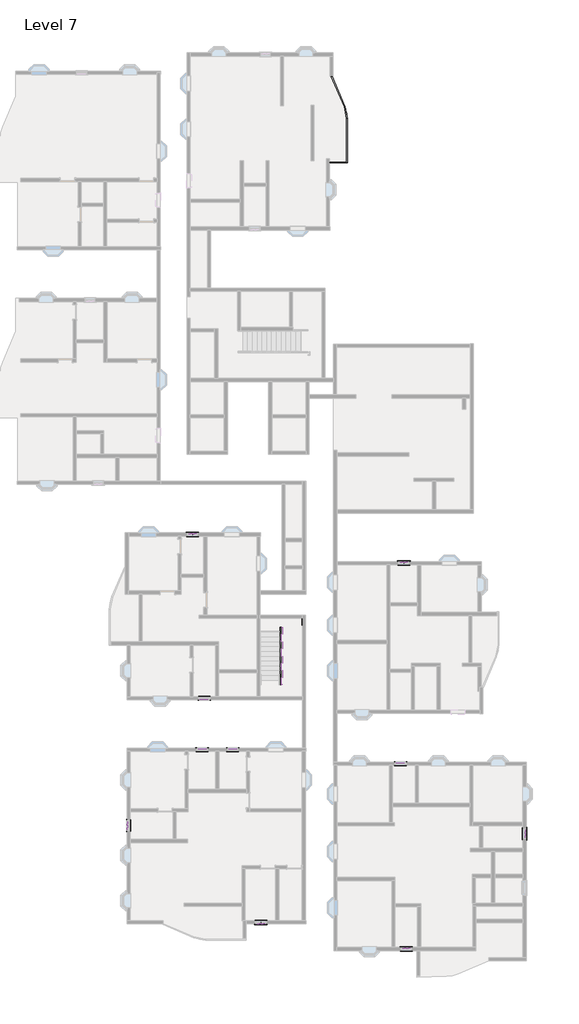
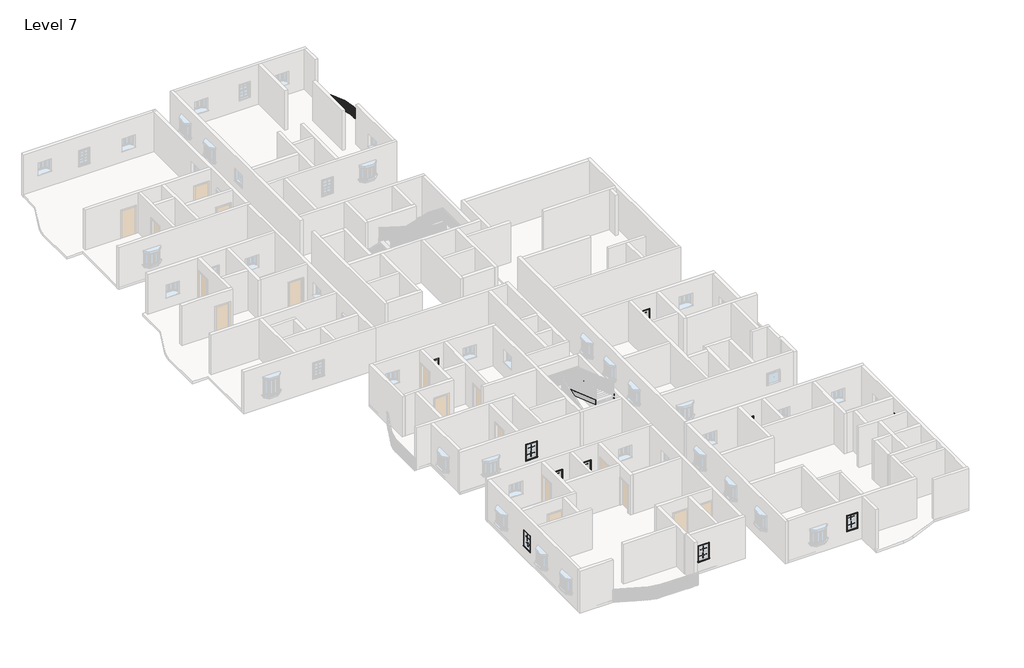
# One storey, part 13 of 14: 40 proxies, 6 members, 1 railing.
"""IFC4 building model written with IfcOpenShell, lengths in millimetres."""

from ifc_helpers import new_model, si_unit, frame, origin, place, context, project, spatial, polyline, circle_curve, outline, extrude, transform, mapped, element, save
from ifc_brep_helpers import plane_surface, cylinder_surface, revolved_surface, advanced_brep
from components import muntin_pattern_2x2_muntin_pattern_2x2_c35c595f, trim_window_exterior_flat_with_sill_e38017c9, trim_window_interior_flat_picture_frame_d728ed12

model = new_model("IFC4")

# Units and contexts
model_context = context("Model", 3, world=origin())
ifc_project = project(units=[si_unit("LENGTHUNIT", "METRE", prefix="MILLI")], contexts=[model_context])

# Site, building, storey
site = spatial("IfcSite", under=ifc_project)
building = spatial("IfcBuilding", under=site)
storey = spatial("IfcBuildingStorey", under=building, Name="Level 7", Elevation=18288.0)

# Proxies
placement = place(None, origin())
muntin_pattern_2x2_muntin_pattern_2x2_shape = muntin_pattern_2x2_muntin_pattern_2x2_c35c595f(model_context)
element("IfcBuildingElementProxy", 1, Name="Muntin Pattern_2x2 : Muntin Pattern_2x2", ObjectType="Muntin Pattern_2x2 : Muntin Pattern_2x2", at=placement, inside=storey, context=model_context, shape_type="MappedRepresentation", body=[
    mapped(muntin_pattern_2x2_muntin_pattern_2x2_shape, transform((-8150.287215, -357.5666506, 19758.025), x_axis=(1.0, 0.0, 0.0), y_axis=(0.0, 1.0, 0.0), z_axis=(0.0, 0.0, 1.0))),
])
element("IfcBuildingElementProxy", 2, Name="Muntin Pattern_2x2 : Muntin Pattern_2x2", ObjectType="Muntin Pattern_2x2 : Muntin Pattern_2x2", at=placement, inside=storey, context=model_context, shape_type="MappedRepresentation", body=[
    mapped(muntin_pattern_2x2_muntin_pattern_2x2_shape, transform((-8150.287215, -402.0166506, 19278.6), x_axis=(1.0, 0.0, 0.0), y_axis=(0.0, 1.0, 0.0), z_axis=(0.0, 0.0, 1.0))),
])
element("IfcBuildingElementProxy", 3, Name="Muntin Pattern_2x2 : Muntin Pattern_2x2", ObjectType="Muntin Pattern_2x2 : Muntin Pattern_2x2", at=placement, inside=storey, context=model_context, shape_type="MappedRepresentation", body=[
    mapped(muntin_pattern_2x2_muntin_pattern_2x2_shape, transform((-7397.812215, -10854.1166506, 19758.025), x_axis=(-1.0, 0.0, 0.0), y_axis=(0.0, -1.0, 0.0), z_axis=(0.0, 0.0, 1.0))),
])
element("IfcBuildingElementProxy", 4, Name="Muntin Pattern_2x2 : Muntin Pattern_2x2", ObjectType="Muntin Pattern_2x2 : Muntin Pattern_2x2", at=placement, inside=storey, context=model_context, shape_type="MappedRepresentation", body=[
    mapped(muntin_pattern_2x2_muntin_pattern_2x2_shape, transform((-7397.812215, -10809.6666506, 19278.6), x_axis=(-1.0, 0.0, 0.0), y_axis=(0.0, -1.0, 0.0), z_axis=(0.0, 0.0, 1.0))),
])
element("IfcBuildingElementProxy", 5, Name="Muntin Pattern_2x2 : Muntin Pattern_2x2", ObjectType="Muntin Pattern_2x2 : Muntin Pattern_2x2", at=placement, inside=storey, context=model_context, shape_type="MappedRepresentation", body=[
    mapped(muntin_pattern_2x2_muntin_pattern_2x2_shape, transform((-7540.687215, -13997.3666506, 19758.025), x_axis=(1.0, 0.0, 0.0), y_axis=(0.0, 1.0, 0.0), z_axis=(0.0, 0.0, 1.0))),
])
element("IfcBuildingElementProxy", 6, Name="Muntin Pattern_2x2 : Muntin Pattern_2x2", ObjectType="Muntin Pattern_2x2 : Muntin Pattern_2x2", at=placement, inside=storey, context=model_context, shape_type="MappedRepresentation", body=[
    mapped(muntin_pattern_2x2_muntin_pattern_2x2_shape, transform((-7540.687215, -14041.8166506, 19278.6), x_axis=(1.0, 0.0, 0.0), y_axis=(0.0, 1.0, 0.0), z_axis=(0.0, 0.0, 1.0))),
])
element("IfcBuildingElementProxy", 7, Name="Muntin Pattern_2x2 : Muntin Pattern_2x2", ObjectType="Muntin Pattern_2x2 : Muntin Pattern_2x2", at=placement, inside=storey, context=model_context, shape_type="MappedRepresentation", body=[
    mapped(muntin_pattern_2x2_muntin_pattern_2x2_shape, transform((-5597.587215, -13997.3666506, 19758.025), x_axis=(1.0, 0.0, 0.0), y_axis=(0.0, 1.0, 0.0), z_axis=(0.0, 0.0, 1.0))),
])
element("IfcBuildingElementProxy", 8, Name="Muntin Pattern_2x2 : Muntin Pattern_2x2", ObjectType="Muntin Pattern_2x2 : Muntin Pattern_2x2", at=placement, inside=storey, context=model_context, shape_type="MappedRepresentation", body=[
    mapped(muntin_pattern_2x2_muntin_pattern_2x2_shape, transform((-5597.587215, -14041.8166506, 19278.6), x_axis=(1.0, 0.0, 0.0), y_axis=(0.0, 1.0, 0.0), z_axis=(0.0, 0.0, 1.0))),
])
element("IfcBuildingElementProxy", 9, Name="Muntin Pattern_2x2 : Muntin Pattern_2x2", ObjectType="Muntin Pattern_2x2 : Muntin Pattern_2x2", at=placement, inside=storey, context=model_context, shape_type="MappedRepresentation", body=[
    mapped(muntin_pattern_2x2_muntin_pattern_2x2_shape, transform((-12255.562215, -18863.6994419, 19758.025), x_axis=(0.0, 1.0, 0.0), y_axis=(-1.0, 0.0, 0.0), z_axis=(0.0, 0.0, 1.0))),
])
element("IfcBuildingElementProxy", 10, Name="Muntin Pattern_2x2 : Muntin Pattern_2x2", ObjectType="Muntin Pattern_2x2 : Muntin Pattern_2x2", at=placement, inside=storey, context=model_context, shape_type="MappedRepresentation", body=[
    mapped(muntin_pattern_2x2_muntin_pattern_2x2_shape, transform((-12211.112215, -18863.6994419, 19278.6), x_axis=(0.0, 1.0, 0.0), y_axis=(-1.0, 0.0, 0.0), z_axis=(0.0, 0.0, 1.0))),
])
element("IfcBuildingElementProxy", 11, Name="Muntin Pattern_2x2 : Muntin Pattern_2x2", ObjectType="Muntin Pattern_2x2 : Muntin Pattern_2x2", at=placement, inside=storey, context=model_context, shape_type="MappedRepresentation", body=[
    mapped(muntin_pattern_2x2_muntin_pattern_2x2_shape, transform((-3806.2891351, -25065.4166506, 19758.025), x_axis=(-1.0, 0.0, 0.0), y_axis=(0.0, -1.0, 0.0), z_axis=(0.0, 0.0, 1.0))),
])
element("IfcBuildingElementProxy", 12, Name="Muntin Pattern_2x2 : Muntin Pattern_2x2", ObjectType="Muntin Pattern_2x2 : Muntin Pattern_2x2", at=placement, inside=storey, context=model_context, shape_type="MappedRepresentation", body=[
    mapped(muntin_pattern_2x2_muntin_pattern_2x2_shape, transform((-3806.2891351, -25020.9666506, 19278.6), x_axis=(-1.0, 0.0, 0.0), y_axis=(0.0, -1.0, 0.0), z_axis=(0.0, 0.0, 1.0))),
])
element("IfcBuildingElementProxy", 13, Name="Muntin Pattern_2x2 : Muntin Pattern_2x2", ObjectType="Muntin Pattern_2x2 : Muntin Pattern_2x2", at=placement, inside=storey, context=model_context, shape_type="MappedRepresentation", body=[
    mapped(muntin_pattern_2x2_muntin_pattern_2x2_shape, transform((5410.0380523, -26615.6292694, 19758.025), x_axis=(1.0, 0.0, 0.0), y_axis=(0.0, 1.0, 0.0), z_axis=(0.0, 0.0, 1.0))),
])
element("IfcBuildingElementProxy", 14, Name="Muntin Pattern_2x2 : Muntin Pattern_2x2", ObjectType="Muntin Pattern_2x2 : Muntin Pattern_2x2", at=placement, inside=storey, context=model_context, shape_type="MappedRepresentation", body=[
    mapped(muntin_pattern_2x2_muntin_pattern_2x2_shape, transform((5410.0380523, -26660.0792694, 19278.6), x_axis=(1.0, 0.0, 0.0), y_axis=(0.0, 1.0, 0.0), z_axis=(0.0, 0.0, 1.0))),
])
element("IfcBuildingElementProxy", 15, Name="Muntin Pattern_2x2 : Muntin Pattern_2x2", ObjectType="Muntin Pattern_2x2 : Muntin Pattern_2x2", at=placement, inside=storey, context=model_context, shape_type="MappedRepresentation", body=[
    mapped(muntin_pattern_2x2_muntin_pattern_2x2_shape, transform((12982.4130523, -19379.8042694, 19758.025), x_axis=(0.0, -1.0, 0.0), y_axis=(1.0, 0.0, 0.0), z_axis=(0.0, 0.0, 1.0))),
])
element("IfcBuildingElementProxy", 16, Name="Muntin Pattern_2x2 : Muntin Pattern_2x2", ObjectType="Muntin Pattern_2x2 : Muntin Pattern_2x2", at=placement, inside=storey, context=model_context, shape_type="MappedRepresentation", body=[
    mapped(muntin_pattern_2x2_muntin_pattern_2x2_shape, transform((12937.9630523, -19379.8042694, 19278.6), x_axis=(0.0, -1.0, 0.0), y_axis=(1.0, 0.0, 0.0), z_axis=(0.0, 0.0, 1.0))),
])
element("IfcBuildingElementProxy", 17, Name="Muntin Pattern_2x2 : Muntin Pattern_2x2", ObjectType="Muntin Pattern_2x2 : Muntin Pattern_2x2", at=placement, inside=storey, context=model_context, shape_type="MappedRepresentation", body=[
    mapped(muntin_pattern_2x2_muntin_pattern_2x2_shape, transform((5048.0880523, -14880.8292694, 19758.025), x_axis=(1.0, 0.0, 0.0), y_axis=(0.0, 1.0, 0.0), z_axis=(0.0, 0.0, 1.0))),
])
element("IfcBuildingElementProxy", 18, Name="Muntin Pattern_2x2 : Muntin Pattern_2x2", ObjectType="Muntin Pattern_2x2 : Muntin Pattern_2x2", at=placement, inside=storey, context=model_context, shape_type="MappedRepresentation", body=[
    mapped(muntin_pattern_2x2_muntin_pattern_2x2_shape, transform((5048.0880523, -14925.2792694, 19278.6), x_axis=(1.0, 0.0, 0.0), y_axis=(0.0, 1.0, 0.0), z_axis=(0.0, 0.0, 1.0))),
])
element("IfcBuildingElementProxy", 19, Name="Muntin Pattern_2x2 : Muntin Pattern_2x2", ObjectType="Muntin Pattern_2x2 : Muntin Pattern_2x2", at=placement, inside=storey, context=model_context, shape_type="MappedRepresentation", body=[
    mapped(muntin_pattern_2x2_muntin_pattern_2x2_shape, transform((5257.6380523, -2168.1292694, 19758.025), x_axis=(1.0, 0.0, 0.0), y_axis=(0.0, 1.0, 0.0), z_axis=(0.0, 0.0, 1.0))),
])
element("IfcBuildingElementProxy", 20, Name="Muntin Pattern_2x2 : Muntin Pattern_2x2", ObjectType="Muntin Pattern_2x2 : Muntin Pattern_2x2", at=placement, inside=storey, context=model_context, shape_type="MappedRepresentation", body=[
    mapped(muntin_pattern_2x2_muntin_pattern_2x2_shape, transform((5257.6380523, -2212.5792694, 19278.6), x_axis=(1.0, 0.0, 0.0), y_axis=(0.0, 1.0, 0.0), z_axis=(0.0, 0.0, 1.0))),
])
trim_window_exterior_flat_with_sill_shape = trim_window_exterior_flat_with_sill_e38017c9(model_context)
element("IfcBuildingElementProxy", 21, Name="Trim-Window-Exterior-Flat : with Sill", ObjectType="Trim-Window-Exterior-Flat : with Sill", at=placement, inside=storey, context=model_context, shape_type="MappedRepresentation", body=[
    mapped(trim_window_exterior_flat_with_sill_shape, transform((-8150.287215, -322.6416506, 20269.2), x_axis=(-1.0, 0.0, 0.0), y_axis=(0.0, 0.0, 1.0), z_axis=(0.0, 1.0, 0.0))),
])
element("IfcBuildingElementProxy", 22, Name="Trim-Window-Exterior-Flat : with Sill", ObjectType="Trim-Window-Exterior-Flat : with Sill", at=placement, inside=storey, context=model_context, shape_type="MappedRepresentation", body=[
    mapped(trim_window_exterior_flat_with_sill_shape, transform((-7397.812215, -10889.0416506, 20269.2), x_axis=(1.0, 0.0, 0.0), y_axis=(0.0, 0.0, 1.0), z_axis=(0.0, -1.0, 0.0))),
])
element("IfcBuildingElementProxy", 23, Name="Trim-Window-Exterior-Flat : with Sill", ObjectType="Trim-Window-Exterior-Flat : with Sill", at=placement, inside=storey, context=model_context, shape_type="MappedRepresentation", body=[
    mapped(trim_window_exterior_flat_with_sill_shape, transform((-7540.687215, -13962.4416506, 20269.2), x_axis=(-1.0, 0.0, 0.0), y_axis=(0.0, 0.0, 1.0), z_axis=(0.0, 1.0, 0.0))),
])
element("IfcBuildingElementProxy", 24, Name="Trim-Window-Exterior-Flat : with Sill", ObjectType="Trim-Window-Exterior-Flat : with Sill", at=placement, inside=storey, context=model_context, shape_type="MappedRepresentation", body=[
    mapped(trim_window_exterior_flat_with_sill_shape, transform((-5597.587215, -13962.4416506, 20269.2), x_axis=(-1.0, 0.0, 0.0), y_axis=(0.0, 0.0, 1.0), z_axis=(0.0, 1.0, 0.0))),
])
element("IfcBuildingElementProxy", 25, Name="Trim-Window-Exterior-Flat : with Sill", ObjectType="Trim-Window-Exterior-Flat : with Sill", at=placement, inside=storey, context=model_context, shape_type="MappedRepresentation", body=[
    mapped(trim_window_exterior_flat_with_sill_shape, transform((-12290.487215, -18863.6994419, 20269.2), x_axis=(0.0, -1.0, 0.0), y_axis=(0.0, 0.0, 1.0), z_axis=(-1.0, 0.0, 0.0))),
])
element("IfcBuildingElementProxy", 26, Name="Trim-Window-Exterior-Flat : with Sill", ObjectType="Trim-Window-Exterior-Flat : with Sill", at=placement, inside=storey, context=model_context, shape_type="MappedRepresentation", body=[
    mapped(trim_window_exterior_flat_with_sill_shape, transform((-3806.2891351, -25100.3416506, 20269.2), x_axis=(1.0, 0.0, 0.0), y_axis=(0.0, 0.0, 1.0), z_axis=(0.0, -1.0, 0.0))),
])
element("IfcBuildingElementProxy", 27, Name="Trim-Window-Exterior-Flat : with Sill", ObjectType="Trim-Window-Exterior-Flat : with Sill", at=placement, inside=storey, context=model_context, shape_type="MappedRepresentation", body=[
    mapped(trim_window_exterior_flat_with_sill_shape, transform((5410.0380523, -26580.7042694, 20269.2), x_axis=(-1.0, 0.0, 0.0), y_axis=(0.0, 0.0, 1.0), z_axis=(0.0, 1.0, 0.0))),
])
element("IfcBuildingElementProxy", 28, Name="Trim-Window-Exterior-Flat : with Sill", ObjectType="Trim-Window-Exterior-Flat : with Sill", at=placement, inside=storey, context=model_context, shape_type="MappedRepresentation", body=[
    mapped(trim_window_exterior_flat_with_sill_shape, transform((13017.3380523, -19379.8042694, 20269.2), x_axis=(0.0, 1.0, 0.0), y_axis=(0.0, 0.0, 1.0), z_axis=(1.0, 0.0, 0.0))),
])
element("IfcBuildingElementProxy", 29, Name="Trim-Window-Exterior-Flat : with Sill", ObjectType="Trim-Window-Exterior-Flat : with Sill", at=placement, inside=storey, context=model_context, shape_type="MappedRepresentation", body=[
    mapped(trim_window_exterior_flat_with_sill_shape, transform((5048.0880523, -14845.9042694, 20269.2), x_axis=(-1.0, 0.0, 0.0), y_axis=(0.0, 0.0, 1.0), z_axis=(0.0, 1.0, 0.0))),
])
element("IfcBuildingElementProxy", 30, Name="Trim-Window-Exterior-Flat : with Sill", ObjectType="Trim-Window-Exterior-Flat : with Sill", at=placement, inside=storey, context=model_context, shape_type="MappedRepresentation", body=[
    mapped(trim_window_exterior_flat_with_sill_shape, transform((5257.6380523, -2133.2042694, 20269.2), x_axis=(-1.0, 0.0, 0.0), y_axis=(0.0, 0.0, 1.0), z_axis=(0.0, 1.0, 0.0))),
])
trim_window_interior_flat_picture_frame_shape = trim_window_interior_flat_picture_frame_d728ed12(model_context)
element("IfcBuildingElementProxy", 31, Name="Trim-Window-Interior-Flat : Picture Frame", ObjectType="Trim-Window-Interior-Flat : Picture Frame", at=placement, inside=storey, context=model_context, shape_type="MappedRepresentation", body=[
    mapped(trim_window_interior_flat_picture_frame_shape, transform((-8150.287215, -525.8416506, 20269.2), x_axis=(1.0, 0.0, 0.0), y_axis=(0.0, 0.0, 1.0), z_axis=(0.0, -1.0, 0.0))),
])
element("IfcBuildingElementProxy", 32, Name="Trim-Window-Interior-Flat : Picture Frame", ObjectType="Trim-Window-Interior-Flat : Picture Frame", at=placement, inside=storey, context=model_context, shape_type="MappedRepresentation", body=[
    mapped(trim_window_interior_flat_picture_frame_shape, transform((-7397.812215, -10685.8416506, 20269.2), x_axis=(-1.0, 0.0, 0.0), y_axis=(0.0, 0.0, 1.0), z_axis=(0.0, 1.0, 0.0))),
])
element("IfcBuildingElementProxy", 33, Name="Trim-Window-Interior-Flat : Picture Frame", ObjectType="Trim-Window-Interior-Flat : Picture Frame", at=placement, inside=storey, context=model_context, shape_type="MappedRepresentation", body=[
    mapped(trim_window_interior_flat_picture_frame_shape, transform((-7540.687215, -14165.6416506, 20269.2), x_axis=(1.0, 0.0, 0.0), y_axis=(0.0, 0.0, 1.0), z_axis=(0.0, -1.0, 0.0))),
])
element("IfcBuildingElementProxy", 34, Name="Trim-Window-Interior-Flat : Picture Frame", ObjectType="Trim-Window-Interior-Flat : Picture Frame", at=placement, inside=storey, context=model_context, shape_type="MappedRepresentation", body=[
    mapped(trim_window_interior_flat_picture_frame_shape, transform((-5597.587215, -14165.6416506, 20269.2), x_axis=(1.0, 0.0, 0.0), y_axis=(0.0, 0.0, 1.0), z_axis=(0.0, -1.0, 0.0))),
])
element("IfcBuildingElementProxy", 35, Name="Trim-Window-Interior-Flat : Picture Frame", ObjectType="Trim-Window-Interior-Flat : Picture Frame", at=placement, inside=storey, context=model_context, shape_type="MappedRepresentation", body=[
    mapped(trim_window_interior_flat_picture_frame_shape, transform((-12087.287215, -18863.6994419, 20269.2), x_axis=(0.0, 1.0, 0.0), y_axis=(0.0, 0.0, 1.0), z_axis=(1.0, 0.0, 0.0))),
])
element("IfcBuildingElementProxy", 36, Name="Trim-Window-Interior-Flat : Picture Frame", ObjectType="Trim-Window-Interior-Flat : Picture Frame", at=placement, inside=storey, context=model_context, shape_type="MappedRepresentation", body=[
    mapped(trim_window_interior_flat_picture_frame_shape, transform((-3806.2891351, -24897.1416506, 20269.2), x_axis=(-1.0, 0.0, 0.0), y_axis=(0.0, 0.0, 1.0), z_axis=(0.0, 1.0, 0.0))),
])
element("IfcBuildingElementProxy", 37, Name="Trim-Window-Interior-Flat : Picture Frame", ObjectType="Trim-Window-Interior-Flat : Picture Frame", at=placement, inside=storey, context=model_context, shape_type="MappedRepresentation", body=[
    mapped(trim_window_interior_flat_picture_frame_shape, transform((5410.0380523, -26783.9042694, 20269.2), x_axis=(1.0, 0.0, 0.0), y_axis=(0.0, 0.0, 1.0), z_axis=(0.0, -1.0, 0.0))),
])
element("IfcBuildingElementProxy", 38, Name="Trim-Window-Interior-Flat : Picture Frame", ObjectType="Trim-Window-Interior-Flat : Picture Frame", at=placement, inside=storey, context=model_context, shape_type="MappedRepresentation", body=[
    mapped(trim_window_interior_flat_picture_frame_shape, transform((12814.1380523, -19379.8042694, 20269.2), x_axis=(0.0, -1.0, 0.0), y_axis=(0.0, 0.0, 1.0), z_axis=(-1.0, 0.0, 0.0))),
])
element("IfcBuildingElementProxy", 39, Name="Trim-Window-Interior-Flat : Picture Frame", ObjectType="Trim-Window-Interior-Flat : Picture Frame", at=placement, inside=storey, context=model_context, shape_type="MappedRepresentation", body=[
    mapped(trim_window_interior_flat_picture_frame_shape, transform((5048.0880523, -15049.1042694, 20269.2), x_axis=(1.0, 0.0, 0.0), y_axis=(0.0, 0.0, 1.0), z_axis=(0.0, -1.0, 0.0))),
])
element("IfcBuildingElementProxy", 40, Name="Trim-Window-Interior-Flat : Picture Frame", ObjectType="Trim-Window-Interior-Flat : Picture Frame", at=placement, inside=storey, context=model_context, shape_type="MappedRepresentation", body=[
    mapped(trim_window_interior_flat_picture_frame_shape, transform((5257.6380523, -2336.4042694, 20269.2), x_axis=(1.0, 0.0, 0.0), y_axis=(0.0, 0.0, 1.0), z_axis=(0.0, -1.0, 0.0))),
])

# Members
element("IfcMember", 41, ObjectType="Stringer - 2\" Width", at=placement, inside=storey, context=model_context, shape_type="SweptSolid", body=[
    extrude(outline(polyline([(-9955.5916506, 18288.0), (-9955.5916506, 18479.3592169), (-6325.8738327, 19735.8), (-5713.7916506, 19735.8), (-5713.7916506, 19625.1301656), (-9576.612129, 18288.0), (-9955.5916506, 18288.0)])), frame((-3908.487215, 0.0, 0.0), z_axis=(1.0, 0.0, 0.0), x_axis=(0.0, 1.0, 0.0)), (0.0, 0.0, 1.0), 50.8),
])
element("IfcMember", 42, ObjectType="Stringer - 2\" Width", at=placement, inside=storey, context=model_context, shape_type="SweptSolid", body=[
    extrude(outline(polyline([(-3908.487215, -5713.7916506), (-3908.487215, -5662.9916506), (-1190.687215, -5662.9916506), (-1190.687215, -5713.7916506), (-3908.487215, -5713.7916506)])), frame((0.0, 0.0, 19431.0), z_axis=(0.0, 0.0, 1.0), x_axis=(1.0, 0.0, 0.0)), (0.0, 0.0, 1.0), 304.8),
])
element("IfcMember", 43, ObjectType="Stringer - 2\" Width", at=placement, inside=storey, context=model_context, shape_type="SweptSolid", body=[
    extrude(outline(polyline([(-5662.9916506, 19635.5476784), (-5662.9916506, 19431.0), (-6003.8711722, 19431.0), (-9949.2416506, 20796.7051656), (-9949.2416506, 21119.2496015), (-5662.9916506, 19635.5476784)])), frame((-1190.687215, 0.0, 0.0), z_axis=(1.0, 0.0, 0.0), x_axis=(0.0, 1.0, 0.0)), (0.0, 0.0, 1.0), 50.8),
])
element("IfcMember", 44, ObjectType="Stringer - 2\" Width", at=placement, inside=storey, context=model_context, shape_type="SweptSolid", body=[
    extrude(outline(polyline([(-9955.5916506, 18288.0), (-9955.5916506, 18479.3592169), (-6342.4416506, 19730.0649861), (-6342.4416506, 19407.5205502), (-9576.612129, 18288.0), (-9955.5916506, 18288.0)])), frame((-2593.7381751, 0.0, 0.0), z_axis=(1.0, 0.0, 0.0), x_axis=(0.0, 1.0, 0.0)), (0.0, 0.0, 1.0), 50.8),
])
element("IfcMember", 45, ObjectType="Stringer - 2\" Width", at=placement, inside=storey, context=model_context, shape_type="SweptSolid", body=[
    extrude(outline(polyline([(-2593.7381751, -6342.4416506), (-2593.7381751, -6291.6416506), (-2492.1381751, -6291.6416506), (-2492.1381751, -6342.4416506), (-2593.7381751, -6342.4416506)])), frame((0.0, 0.0, 19431.0), z_axis=(0.0, 0.0, 1.0), x_axis=(1.0, 0.0, 0.0)), (0.0, 0.0, 1.0), 304.8),
])
element("IfcMember", 46, ObjectType="Stringer - 2\" Width", at=placement, inside=storey, context=model_context, shape_type="SweptSolid", body=[
    extrude(outline(polyline([(-6291.6416506, 19853.1572938), (-6291.6416506, 19530.6128579), (-9949.2416506, 20796.7051656), (-9949.2416506, 21119.2496015), (-6291.6416506, 19853.1572938)])), frame((-2492.1381751, 0.0, 0.0), z_axis=(1.0, 0.0, 0.0), x_axis=(0.0, 1.0, 0.0)), (0.0, 0.0, 1.0), 50.8),
])

# Railing
element("IfcRailing", 47, ObjectType="Handrail - Rectangular", at=placement, inside=storey, context=model_context, shape_type="SolidModel", body=[
    advanced_brep(
    [(549.8108649, 23180.4215905, 19202.4), (549.8108649, 23180.4215905, 19151.6), (549.8108649, 23129.6215905, 19151.6), (549.8108649, 23129.6215905, 19202.4), (1629.3108649, 23180.4215905, 19202.4), (1629.3108649, 23180.4215905, 19151.6), (1680.1108649, 23129.6215905, 19151.6), (1680.1108649, 23129.6215905, 19202.4), (1629.3108649, 25921.9580583, 19202.4), (1629.3108649, 25921.9580583, 19151.6), (1680.1108649, 25921.9580583, 19151.6), (1680.1108649, 25921.9580583, 19202.4), (1475.5051478, 26671.8537734, 19151.6), (1475.5051478, 26671.8537734, 19202.4), (1522.203662, 26691.8509925, 19151.6), (1522.203662, 26691.8509925, 19202.4), (640.7616078, 28621.188975, 19202.4), (687.460122, 28641.186194, 19202.4), (687.460122, 28641.186194, 19151.6), (640.7616078, 28621.188975, 19151.6)],
    [
        (0, 1),
        (1, 2),
        (2, 3),
        (3, 0),
        (0, 4),
        (4, 5),
        (5, 1),
        (5, 6),
        (6, 2),
        (6, 7),
        (7, 3),
        (7, 4),
        (4, 8),
        (8, 9),
        (9, 5),
        (9, 10),
        (10, 6),
        (10, 11),
        (11, 7),
        (11, 8),
        (12, 9, circle_curve(frame((-275.6891351, 25921.9580583, 19151.6), z_axis=(0.0, 0.0, -1.0), x_axis=(1.0, 0.0, 0.0)), 1905.0)),
        (8, 13, circle_curve(frame((-275.6891351, 25921.9580583, 19202.4), z_axis=(0.0, 0.0, 1.0), x_axis=(1.0, 0.0, 0.0)), 1905.0)),
        (13, 12),
        (14, 10, circle_curve(frame((-275.6891351, 25921.9580583, 19151.6), z_axis=(0.0, 0.0, -1.0), x_axis=(1.0, 0.0, 0.0)), 1955.8)),
        (12, 14),
        (15, 11, circle_curve(frame((-275.6891351, 25921.9580583, 19202.4), z_axis=(0.0, 0.0, -1.0), x_axis=(1.0, 0.0, 0.0)), 1955.8)),
        (14, 15),
        (15, 13),
        (16, 17),
        (17, 18),
        (18, 19),
        (19, 16),
        (13, 16),
        (19, 12),
        (18, 14),
        (17, 15),
    ],
    [
        plane_surface(frame((549.8108649, 23155.0215905, 19202.4), z_axis=(-1.0, 0.0, 0.0), x_axis=(0.0, 1.0, 0.0))),
        plane_surface(frame((549.8108649, 23180.4215905, 19202.4), z_axis=(0.0, 1.0, 0.0), x_axis=(1.0, 0.0, 0.0))),
        plane_surface(frame((549.8108649, 23180.4215905, 19151.6), z_axis=(0.0, 0.0, -1.0), x_axis=(1.0, 0.0, 0.0))),
        plane_surface(frame((549.8108649, 23129.6215905, 19151.6), z_axis=(0.0, -1.0, 0.0), x_axis=(1.0, 0.0, 0.0))),
        plane_surface(frame((549.8108649, 23129.6215905, 19202.4), z_axis=(0.0, 0.0, 1.0), x_axis=(1.0, 0.0, 0.0))),
        plane_surface(frame((1629.3108649, 23180.4215905, 19202.4), z_axis=(-1.0, 0.0, 0.0), x_axis=(0.0, 1.0, 0.0))),
        plane_surface(frame((1629.3108649, 23180.4215905, 19151.6), z_axis=(0.0, 0.0, -1.0), x_axis=(0.0, 1.0, 0.0))),
        plane_surface(frame((1680.1108649, 23129.6215905, 19151.6), z_axis=(1.0, 0.0, 0.0), x_axis=(0.0, 1.0, 0.0))),
        plane_surface(frame((1680.1108649, 23129.6215905, 19202.4), z_axis=(0.0, 0.0, 1.0), x_axis=(0.0, 1.0, 0.0))),
        revolved_surface(polyline([(1629.3108649, 25921.9580583, 19202.4), (1629.3108649, 25921.9580583, 19151.6)]), (-275.6891351, 25921.9580583, 19202.4), (0.0, 0.0, 1.0)),
        plane_surface(frame((-275.6891351, 25921.9580583, 19151.6), z_axis=(0.0, 0.0, -1.0), x_axis=(1.0, 0.0, 0.0))),
        cylinder_surface(frame((-275.6891351, 25921.9580583, 19202.4), z_axis=(0.0, 0.0, 1.0), x_axis=(1.0, 0.0, 0.0)), 1955.8),
        plane_surface(frame((-275.6891351, 25921.9580583, 19202.4), z_axis=(0.0, 0.0, 1.0), x_axis=(1.0, 0.0, 0.0))),
        plane_surface(frame((664.1108649, 28631.1875845, 19202.4), z_axis=(-0.39364604467361036, 0.91926209076238, 0.0), x_axis=(0.91926209076238, 0.39364604467361036, 0.0))),
        plane_surface(frame((1475.5051478, 26671.8537734, 19202.4), z_axis=(-0.91926209076238, -0.3936460446736102, 0.0), x_axis=(-0.3936460446736102, 0.91926209076238, 0.0))),
        plane_surface(frame((1475.5051478, 26671.8537734, 19151.6), z_axis=(0.0, 0.0, -1.0), x_axis=(-0.3936460446736102, 0.91926209076238, 0.0))),
        plane_surface(frame((1522.203662, 26691.8509925, 19151.6), z_axis=(0.91926209076238, 0.3936460446736102, 0.0), x_axis=(-0.3936460446736102, 0.91926209076238, 0.0))),
        plane_surface(frame((1522.203662, 26691.8509925, 19202.4), z_axis=(0.0, 0.0, 1.0), x_axis=(-0.3936460446736102, 0.91926209076238, 0.0))),
    ],
    [
        (0, [[1, 2, 3, 4]]),
        (1, [[-1, 5, 6, 7]]),
        (2, [[-2, -7, 8, 9]]),
        (3, [[-3, -9, 10, 11]]),
        (4, [[-4, -11, 12, -5]]),
        (5, [[-6, 13, 14, 15]]),
        (6, [[-8, -15, 16, 17]]),
        (7, [[-10, -17, 18, 19]]),
        (8, [[-12, -19, 20, -13]]),
        (9, [[21, -14, 22, 23]]),
        (10, [[24, -16, -21, 25]]),
        (11, [[26, -18, -24, 27]]),
        (12, [[-22, -20, -26, 28]]),
        (13, [[29, 30, 31, 32]]),
        (14, [[-23, 33, -32, 34]]),
        (15, [[-25, -34, -31, 35]]),
        (16, [[-27, -35, -30, 36]]),
        (17, [[-28, -36, -29, -33]]),
    ],
),
    extrude(outline(polyline([(711.4710921, 28544.7864585), (693.9591493, 28537.2875014), (686.4601921, 28554.7994442), (703.9721349, 28562.2984014), (711.4710921, 28544.7864585)])), frame((0.0, 0.0, 18288.0), z_axis=(0.0, 0.0, 1.0), x_axis=(1.0, 0.0, 0.0)), (0.0, 0.0, 1.0), 863.6),
    extrude(outline(polyline([(751.4655302, 28451.3894301), (733.9535874, 28443.890473), (726.4546303, 28461.4024158), (743.9665731, 28468.9013729), (751.4655302, 28451.3894301)])), frame((0.0, 0.0, 18288.0), z_axis=(0.0, 0.0, 1.0), x_axis=(1.0, 0.0, 0.0)), (0.0, 0.0, 1.0), 863.6),
    extrude(outline(polyline([(791.4599684, 28357.9924017), (773.9480255, 28350.4934445), (766.4490684, 28368.0053874), (783.9610112, 28375.5043445), (791.4599684, 28357.9924017)])), frame((0.0, 0.0, 18288.0), z_axis=(0.0, 0.0, 1.0), x_axis=(1.0, 0.0, 0.0)), (0.0, 0.0, 1.0), 863.6),
    extrude(outline(polyline([(831.4544065, 28264.5953733), (813.9424637, 28257.0964161), (806.4435065, 28274.608359), (823.9554494, 28282.1073161), (831.4544065, 28264.5953733)])), frame((0.0, 0.0, 18288.0), z_axis=(0.0, 0.0, 1.0), x_axis=(1.0, 0.0, 0.0)), (0.0, 0.0, 1.0), 863.6),
    extrude(outline(polyline([(871.4488446, 28171.1983449), (853.9369018, 28163.6993877), (846.4379447, 28181.2113305), (863.9498875, 28188.7102877), (871.4488446, 28171.1983449)])), frame((0.0, 0.0, 18288.0), z_axis=(0.0, 0.0, 1.0), x_axis=(1.0, 0.0, 0.0)), (0.0, 0.0, 1.0), 863.6),
    extrude(outline(polyline([(911.4432828, 28077.8013164), (893.93134, 28070.3023593), (886.4323828, 28087.8143021), (903.9443256, 28095.3132593), (911.4432828, 28077.8013164)])), frame((0.0, 0.0, 18288.0), z_axis=(0.0, 0.0, 1.0), x_axis=(1.0, 0.0, 0.0)), (0.0, 0.0, 1.0), 863.6),
    extrude(outline(polyline([(951.4377209, 27984.404288), (933.9257781, 27976.9053309), (926.4268209, 27994.4172737), (943.9387638, 28001.9162308), (951.4377209, 27984.404288)])), frame((0.0, 0.0, 18288.0), z_axis=(0.0, 0.0, 1.0), x_axis=(1.0, 0.0, 0.0)), (0.0, 0.0, 1.0), 863.6),
    extrude(outline(polyline([(991.4321591, 27891.0072596), (973.9202162, 27883.5083024), (966.4212591, 27901.0202453), (983.9332019, 27908.5192024), (991.4321591, 27891.0072596)])), frame((0.0, 0.0, 18288.0), z_axis=(0.0, 0.0, 1.0), x_axis=(1.0, 0.0, 0.0)), (0.0, 0.0, 1.0), 863.6),
    extrude(outline(polyline([(1031.4265972, 27797.6102312), (1013.9146544, 27790.111274), (1006.4156972, 27807.6232168), (1023.9276401, 27815.122174), (1031.4265972, 27797.6102312)])), frame((0.0, 0.0, 18288.0), z_axis=(0.0, 0.0, 1.0), x_axis=(1.0, 0.0, 0.0)), (0.0, 0.0, 1.0), 863.6),
    extrude(outline(polyline([(1071.4210353, 27704.2132027), (1053.9090925, 27696.7142456), (1046.4101354, 27714.2261884), (1063.9220782, 27721.7251456), (1071.4210353, 27704.2132027)])), frame((0.0, 0.0, 18288.0), z_axis=(0.0, 0.0, 1.0), x_axis=(1.0, 0.0, 0.0)), (0.0, 0.0, 1.0), 863.6),
    extrude(outline(polyline([(1111.4154735, 27610.8161743), (1093.9035307, 27603.3172172), (1086.4045735, 27620.82916), (1103.9165163, 27628.3281172), (1111.4154735, 27610.8161743)])), frame((0.0, 0.0, 18288.0), z_axis=(0.0, 0.0, 1.0), x_axis=(1.0, 0.0, 0.0)), (0.0, 0.0, 1.0), 863.6),
    extrude(outline(polyline([(1151.4099116, 27517.4191459), (1133.8979688, 27509.9201888), (1126.3990116, 27527.4321316), (1143.9109545, 27534.9310887), (1151.4099116, 27517.4191459)])), frame((0.0, 0.0, 18288.0), z_axis=(0.0, 0.0, 1.0), x_axis=(1.0, 0.0, 0.0)), (0.0, 0.0, 1.0), 863.6),
    extrude(outline(polyline([(1191.4043498, 27424.0221175), (1173.8924069, 27416.5231603), (1166.3934498, 27434.0351032), (1183.9053926, 27441.5340603), (1191.4043498, 27424.0221175)])), frame((0.0, 0.0, 18288.0), z_axis=(0.0, 0.0, 1.0), x_axis=(1.0, 0.0, 0.0)), (0.0, 0.0, 1.0), 863.6),
    extrude(outline(polyline([(1231.3987879, 27330.6250891), (1213.8868451, 27323.1261319), (1206.3878879, 27340.6380747), (1223.8998307, 27348.1370319), (1231.3987879, 27330.6250891)])), frame((0.0, 0.0, 18288.0), z_axis=(0.0, 0.0, 1.0), x_axis=(1.0, 0.0, 0.0)), (0.0, 0.0, 1.0), 863.6),
    extrude(outline(polyline([(1271.393226, 27237.2280606), (1253.8812832, 27229.7291035), (1246.3823261, 27247.2410463), (1263.8942689, 27254.7400035), (1271.393226, 27237.2280606)])), frame((0.0, 0.0, 18288.0), z_axis=(0.0, 0.0, 1.0), x_axis=(1.0, 0.0, 0.0)), (0.0, 0.0, 1.0), 863.6),
    extrude(outline(polyline([(1311.3876642, 27143.8310322), (1293.8757213, 27136.3320751), (1286.3767642, 27153.8440179), (1303.888707, 27161.342975), (1311.3876642, 27143.8310322)])), frame((0.0, 0.0, 18288.0), z_axis=(0.0, 0.0, 1.0), x_axis=(1.0, 0.0, 0.0)), (0.0, 0.0, 1.0), 863.6),
    extrude(outline(polyline([(1351.3821023, 27050.4340038), (1333.8701595, 27042.9350466), (1326.3712023, 27060.4469895), (1343.8831452, 27067.9459466), (1351.3821023, 27050.4340038)])), frame((0.0, 0.0, 18288.0), z_axis=(0.0, 0.0, 1.0), x_axis=(1.0, 0.0, 0.0)), (0.0, 0.0, 1.0), 863.6),
    extrude(outline(polyline([(1391.3765405, 26957.0369754), (1373.8645976, 26949.5380182), (1366.3656405, 26967.0499611), (1383.8775833, 26974.5489182), (1391.3765405, 26957.0369754)])), frame((0.0, 0.0, 18288.0), z_axis=(0.0, 0.0, 1.0), x_axis=(1.0, 0.0, 0.0)), (0.0, 0.0, 1.0), 863.6),
    extrude(outline(polyline([(1431.3709786, 26863.639947), (1413.8590358, 26856.1409898), (1406.3600786, 26873.6529326), (1423.8720214, 26881.1518898), (1431.3709786, 26863.639947)])), frame((0.0, 0.0, 18288.0), z_axis=(0.0, 0.0, 1.0), x_axis=(1.0, 0.0, 0.0)), (0.0, 0.0, 1.0), 863.6),
    extrude(outline(polyline([(1471.3654167, 26770.2429185), (1453.8534739, 26762.7439614), (1446.3545168, 26780.2559042), (1463.8664596, 26787.7548614), (1471.3654167, 26770.2429185)])), frame((0.0, 0.0, 18288.0), z_axis=(0.0, 0.0, 1.0), x_axis=(1.0, 0.0, 0.0)), (0.0, 0.0, 1.0), 863.6),
    extrude(outline(polyline([(1537.4917391, 26611.722401), (1519.7200483, 26604.8616791), (1512.8593263, 26622.6333699), (1530.6310171, 26629.4940918), (1537.4917391, 26611.722401)])), frame((0.0, 0.0, 18288.0), z_axis=(0.0, 0.0, 1.0), x_axis=(1.0, 0.0, 0.0)), (0.0, 0.0, 1.0), 863.6),
    extrude(outline(polyline([(1571.2676162, 26515.3807493), (1553.1596103, 26509.4644479), (1547.2433088, 26527.5724538), (1565.3513147, 26533.4887552), (1571.2676162, 26515.3807493)])), frame((0.0, 0.0, 18288.0), z_axis=(0.0, 0.0, 1.0), x_axis=(1.0, 0.0, 0.0)), (0.0, 0.0, 1.0), 863.6),
    extrude(outline(polyline([(1599.9284504, 26417.3956468), (1581.5342785, 26412.4401508), (1576.5787825, 26430.8343227), (1594.9729544, 26435.7898187), (1599.9284504, 26417.3956468)])), frame((0.0, 0.0, 18288.0), z_axis=(0.0, 0.0, 1.0), x_axis=(1.0, 0.0, 0.0)), (0.0, 0.0, 1.0), 863.6),
    extrude(outline(polyline([(1623.3948673, 26318.0384578), (1604.7654711, 26314.0574912), (1600.7845045, 26332.6868874), (1619.4139008, 26336.667854), (1623.3948673, 26318.0384578)])), frame((0.0, 0.0, 18288.0), z_axis=(0.0, 0.0, 1.0), x_axis=(1.0, 0.0, 0.0)), (0.0, 0.0, 1.0), 863.6),
    extrude(outline(polyline([(1641.601878, 26217.5843464), (1622.7888504, 26214.5889343), (1619.7934383, 26233.4019618), (1638.6064659, 26236.3973739), (1641.601878, 26217.5843464)])), frame((0.0, 0.0, 18288.0), z_axis=(0.0, 0.0, 1.0), x_axis=(1.0, 0.0, 0.0)), (0.0, 0.0, 1.0), 863.6),
    extrude(outline(polyline([(1654.4990591, 26116.3115146), (1635.5545019, 26114.3099526), (1633.5529398, 26133.2545098), (1652.4974971, 26135.2560719), (1654.4990591, 26116.3115146)])), frame((0.0, 0.0, 18288.0), z_axis=(0.0, 0.0, 1.0), x_axis=(1.0, 0.0, 0.0)), (0.0, 0.0, 1.0), 863.6),
    extrude(outline(polyline([(1662.0506927, 26014.5004319), (1643.0270716, 26013.4982632), (1642.0249029, 26032.5218842), (1661.048524, 26033.524053), (1662.0506927, 26014.5004319)])), frame((0.0, 0.0, 18288.0), z_axis=(0.0, 0.0, 1.0), x_axis=(1.0, 0.0, 0.0)), (0.0, 0.0, 1.0), 863.6),
    extrude(outline(polyline([(1664.2358649, 25888.6965905), (1645.1858649, 25888.6965905), (1645.1858649, 25907.7465905), (1664.2358649, 25907.7465905), (1664.2358649, 25888.6965905)])), frame((0.0, 0.0, 18288.0), z_axis=(0.0, 0.0, 1.0), x_axis=(1.0, 0.0, 0.0)), (0.0, 0.0, 1.0), 863.6),
    extrude(outline(polyline([(1664.2358649, 25787.0965905), (1645.1858649, 25787.0965905), (1645.1858649, 25806.1465905), (1664.2358649, 25806.1465905), (1664.2358649, 25787.0965905)])), frame((0.0, 0.0, 18288.0), z_axis=(0.0, 0.0, 1.0), x_axis=(1.0, 0.0, 0.0)), (0.0, 0.0, 1.0), 863.6),
    extrude(outline(polyline([(1664.2358649, 25685.4965905), (1645.1858649, 25685.4965905), (1645.1858649, 25704.5465905), (1664.2358649, 25704.5465905), (1664.2358649, 25685.4965905)])), frame((0.0, 0.0, 18288.0), z_axis=(0.0, 0.0, 1.0), x_axis=(1.0, 0.0, 0.0)), (0.0, 0.0, 1.0), 863.6),
    extrude(outline(polyline([(1664.2358649, 25583.8965905), (1645.1858649, 25583.8965905), (1645.1858649, 25602.9465905), (1664.2358649, 25602.9465905), (1664.2358649, 25583.8965905)])), frame((0.0, 0.0, 18288.0), z_axis=(0.0, 0.0, 1.0), x_axis=(1.0, 0.0, 0.0)), (0.0, 0.0, 1.0), 863.6),
    extrude(outline(polyline([(1664.2358649, 25482.2965905), (1645.1858649, 25482.2965905), (1645.1858649, 25501.3465905), (1664.2358649, 25501.3465905), (1664.2358649, 25482.2965905)])), frame((0.0, 0.0, 18288.0), z_axis=(0.0, 0.0, 1.0), x_axis=(1.0, 0.0, 0.0)), (0.0, 0.0, 1.0), 863.6),
    extrude(outline(polyline([(1664.2358649, 25380.6965905), (1645.1858649, 25380.6965905), (1645.1858649, 25399.7465905), (1664.2358649, 25399.7465905), (1664.2358649, 25380.6965905)])), frame((0.0, 0.0, 18288.0), z_axis=(0.0, 0.0, 1.0), x_axis=(1.0, 0.0, 0.0)), (0.0, 0.0, 1.0), 863.6),
    extrude(outline(polyline([(1664.2358649, 25279.0965905), (1645.1858649, 25279.0965905), (1645.1858649, 25298.1465905), (1664.2358649, 25298.1465905), (1664.2358649, 25279.0965905)])), frame((0.0, 0.0, 18288.0), z_axis=(0.0, 0.0, 1.0), x_axis=(1.0, 0.0, 0.0)), (0.0, 0.0, 1.0), 863.6),
    extrude(outline(polyline([(1664.2358649, 25177.4965905), (1645.1858649, 25177.4965905), (1645.1858649, 25196.5465905), (1664.2358649, 25196.5465905), (1664.2358649, 25177.4965905)])), frame((0.0, 0.0, 18288.0), z_axis=(0.0, 0.0, 1.0), x_axis=(1.0, 0.0, 0.0)), (0.0, 0.0, 1.0), 863.6),
    extrude(outline(polyline([(1664.2358649, 25075.8965905), (1645.1858649, 25075.8965905), (1645.1858649, 25094.9465905), (1664.2358649, 25094.9465905), (1664.2358649, 25075.8965905)])), frame((0.0, 0.0, 18288.0), z_axis=(0.0, 0.0, 1.0), x_axis=(1.0, 0.0, 0.0)), (0.0, 0.0, 1.0), 863.6),
    extrude(outline(polyline([(1664.2358649, 24974.2965905), (1645.1858649, 24974.2965905), (1645.1858649, 24993.3465905), (1664.2358649, 24993.3465905), (1664.2358649, 24974.2965905)])), frame((0.0, 0.0, 18288.0), z_axis=(0.0, 0.0, 1.0), x_axis=(1.0, 0.0, 0.0)), (0.0, 0.0, 1.0), 863.6),
    extrude(outline(polyline([(1664.2358649, 24872.6965905), (1645.1858649, 24872.6965905), (1645.1858649, 24891.7465905), (1664.2358649, 24891.7465905), (1664.2358649, 24872.6965905)])), frame((0.0, 0.0, 18288.0), z_axis=(0.0, 0.0, 1.0), x_axis=(1.0, 0.0, 0.0)), (0.0, 0.0, 1.0), 863.6),
    extrude(outline(polyline([(1664.2358649, 24771.0965905), (1645.1858649, 24771.0965905), (1645.1858649, 24790.1465905), (1664.2358649, 24790.1465905), (1664.2358649, 24771.0965905)])), frame((0.0, 0.0, 18288.0), z_axis=(0.0, 0.0, 1.0), x_axis=(1.0, 0.0, 0.0)), (0.0, 0.0, 1.0), 863.6),
    extrude(outline(polyline([(1664.2358649, 24669.4965905), (1645.1858649, 24669.4965905), (1645.1858649, 24688.5465905), (1664.2358649, 24688.5465905), (1664.2358649, 24669.4965905)])), frame((0.0, 0.0, 18288.0), z_axis=(0.0, 0.0, 1.0), x_axis=(1.0, 0.0, 0.0)), (0.0, 0.0, 1.0), 863.6),
    extrude(outline(polyline([(1664.2358649, 24567.8965905), (1645.1858649, 24567.8965905), (1645.1858649, 24586.9465905), (1664.2358649, 24586.9465905), (1664.2358649, 24567.8965905)])), frame((0.0, 0.0, 18288.0), z_axis=(0.0, 0.0, 1.0), x_axis=(1.0, 0.0, 0.0)), (0.0, 0.0, 1.0), 863.6),
    extrude(outline(polyline([(1664.2358649, 24466.2965905), (1645.1858649, 24466.2965905), (1645.1858649, 24485.3465905), (1664.2358649, 24485.3465905), (1664.2358649, 24466.2965905)])), frame((0.0, 0.0, 18288.0), z_axis=(0.0, 0.0, 1.0), x_axis=(1.0, 0.0, 0.0)), (0.0, 0.0, 1.0), 863.6),
    extrude(outline(polyline([(1664.2358649, 24364.6965905), (1645.1858649, 24364.6965905), (1645.1858649, 24383.7465905), (1664.2358649, 24383.7465905), (1664.2358649, 24364.6965905)])), frame((0.0, 0.0, 18288.0), z_axis=(0.0, 0.0, 1.0), x_axis=(1.0, 0.0, 0.0)), (0.0, 0.0, 1.0), 863.6),
    extrude(outline(polyline([(1664.2358649, 24263.0965905), (1645.1858649, 24263.0965905), (1645.1858649, 24282.1465905), (1664.2358649, 24282.1465905), (1664.2358649, 24263.0965905)])), frame((0.0, 0.0, 18288.0), z_axis=(0.0, 0.0, 1.0), x_axis=(1.0, 0.0, 0.0)), (0.0, 0.0, 1.0), 863.6),
    extrude(outline(polyline([(1664.2358649, 24161.4965905), (1645.1858649, 24161.4965905), (1645.1858649, 24180.5465905), (1664.2358649, 24180.5465905), (1664.2358649, 24161.4965905)])), frame((0.0, 0.0, 18288.0), z_axis=(0.0, 0.0, 1.0), x_axis=(1.0, 0.0, 0.0)), (0.0, 0.0, 1.0), 863.6),
    extrude(outline(polyline([(1664.2358649, 24059.8965905), (1645.1858649, 24059.8965905), (1645.1858649, 24078.9465905), (1664.2358649, 24078.9465905), (1664.2358649, 24059.8965905)])), frame((0.0, 0.0, 18288.0), z_axis=(0.0, 0.0, 1.0), x_axis=(1.0, 0.0, 0.0)), (0.0, 0.0, 1.0), 863.6),
    extrude(outline(polyline([(1664.2358649, 23958.2965905), (1645.1858649, 23958.2965905), (1645.1858649, 23977.3465905), (1664.2358649, 23977.3465905), (1664.2358649, 23958.2965905)])), frame((0.0, 0.0, 18288.0), z_axis=(0.0, 0.0, 1.0), x_axis=(1.0, 0.0, 0.0)), (0.0, 0.0, 1.0), 863.6),
    extrude(outline(polyline([(1664.2358649, 23856.6965905), (1645.1858649, 23856.6965905), (1645.1858649, 23875.7465905), (1664.2358649, 23875.7465905), (1664.2358649, 23856.6965905)])), frame((0.0, 0.0, 18288.0), z_axis=(0.0, 0.0, 1.0), x_axis=(1.0, 0.0, 0.0)), (0.0, 0.0, 1.0), 863.6),
    extrude(outline(polyline([(1664.2358649, 23755.0965905), (1645.1858649, 23755.0965905), (1645.1858649, 23774.1465905), (1664.2358649, 23774.1465905), (1664.2358649, 23755.0965905)])), frame((0.0, 0.0, 18288.0), z_axis=(0.0, 0.0, 1.0), x_axis=(1.0, 0.0, 0.0)), (0.0, 0.0, 1.0), 863.6),
    extrude(outline(polyline([(1664.2358649, 23653.4965905), (1645.1858649, 23653.4965905), (1645.1858649, 23672.5465905), (1664.2358649, 23672.5465905), (1664.2358649, 23653.4965905)])), frame((0.0, 0.0, 18288.0), z_axis=(0.0, 0.0, 1.0), x_axis=(1.0, 0.0, 0.0)), (0.0, 0.0, 1.0), 863.6),
    extrude(outline(polyline([(1664.2358649, 23551.8965905), (1645.1858649, 23551.8965905), (1645.1858649, 23570.9465905), (1664.2358649, 23570.9465905), (1664.2358649, 23551.8965905)])), frame((0.0, 0.0, 18288.0), z_axis=(0.0, 0.0, 1.0), x_axis=(1.0, 0.0, 0.0)), (0.0, 0.0, 1.0), 863.6),
    extrude(outline(polyline([(1664.2358649, 23450.2965905), (1645.1858649, 23450.2965905), (1645.1858649, 23469.3465905), (1664.2358649, 23469.3465905), (1664.2358649, 23450.2965905)])), frame((0.0, 0.0, 18288.0), z_axis=(0.0, 0.0, 1.0), x_axis=(1.0, 0.0, 0.0)), (0.0, 0.0, 1.0), 863.6),
    extrude(outline(polyline([(1664.2358649, 23348.6965905), (1645.1858649, 23348.6965905), (1645.1858649, 23367.7465905), (1664.2358649, 23367.7465905), (1664.2358649, 23348.6965905)])), frame((0.0, 0.0, 18288.0), z_axis=(0.0, 0.0, 1.0), x_axis=(1.0, 0.0, 0.0)), (0.0, 0.0, 1.0), 863.6),
    extrude(outline(polyline([(1664.2358649, 23247.0965905), (1645.1858649, 23247.0965905), (1645.1858649, 23266.1465905), (1664.2358649, 23266.1465905), (1664.2358649, 23247.0965905)])), frame((0.0, 0.0, 18288.0), z_axis=(0.0, 0.0, 1.0), x_axis=(1.0, 0.0, 0.0)), (0.0, 0.0, 1.0), 863.6),
    extrude(outline(polyline([(1556.2858649, 23145.4965905), (1556.2858649, 23164.5465905), (1575.3358649, 23164.5465905), (1575.3358649, 23145.4965905), (1556.2858649, 23145.4965905)])), frame((0.0, 0.0, 18288.0), z_axis=(0.0, 0.0, 1.0), x_axis=(1.0, 0.0, 0.0)), (0.0, 0.0, 1.0), 863.6),
    extrude(outline(polyline([(1454.6858649, 23145.4965905), (1454.6858649, 23164.5465905), (1473.7358649, 23164.5465905), (1473.7358649, 23145.4965905), (1454.6858649, 23145.4965905)])), frame((0.0, 0.0, 18288.0), z_axis=(0.0, 0.0, 1.0), x_axis=(1.0, 0.0, 0.0)), (0.0, 0.0, 1.0), 863.6),
    extrude(outline(polyline([(1353.0858649, 23145.4965905), (1353.0858649, 23164.5465905), (1372.1358649, 23164.5465905), (1372.1358649, 23145.4965905), (1353.0858649, 23145.4965905)])), frame((0.0, 0.0, 18288.0), z_axis=(0.0, 0.0, 1.0), x_axis=(1.0, 0.0, 0.0)), (0.0, 0.0, 1.0), 863.6),
    extrude(outline(polyline([(1251.4858649, 23145.4965905), (1251.4858649, 23164.5465905), (1270.5358649, 23164.5465905), (1270.5358649, 23145.4965905), (1251.4858649, 23145.4965905)])), frame((0.0, 0.0, 18288.0), z_axis=(0.0, 0.0, 1.0), x_axis=(1.0, 0.0, 0.0)), (0.0, 0.0, 1.0), 863.6),
    extrude(outline(polyline([(1149.8858649, 23145.4965905), (1149.8858649, 23164.5465905), (1168.9358649, 23164.5465905), (1168.9358649, 23145.4965905), (1149.8858649, 23145.4965905)])), frame((0.0, 0.0, 18288.0), z_axis=(0.0, 0.0, 1.0), x_axis=(1.0, 0.0, 0.0)), (0.0, 0.0, 1.0), 863.6),
    extrude(outline(polyline([(1048.2858649, 23145.4965905), (1048.2858649, 23164.5465905), (1067.3358649, 23164.5465905), (1067.3358649, 23145.4965905), (1048.2858649, 23145.4965905)])), frame((0.0, 0.0, 18288.0), z_axis=(0.0, 0.0, 1.0), x_axis=(1.0, 0.0, 0.0)), (0.0, 0.0, 1.0), 863.6),
    extrude(outline(polyline([(946.6858649, 23145.4965905), (946.6858649, 23164.5465905), (965.7358649, 23164.5465905), (965.7358649, 23145.4965905), (946.6858649, 23145.4965905)])), frame((0.0, 0.0, 18288.0), z_axis=(0.0, 0.0, 1.0), x_axis=(1.0, 0.0, 0.0)), (0.0, 0.0, 1.0), 863.6),
    extrude(outline(polyline([(845.0858649, 23145.4965905), (845.0858649, 23164.5465905), (864.1358649, 23164.5465905), (864.1358649, 23145.4965905), (845.0858649, 23145.4965905)])), frame((0.0, 0.0, 18288.0), z_axis=(0.0, 0.0, 1.0), x_axis=(1.0, 0.0, 0.0)), (0.0, 0.0, 1.0), 863.6),
    extrude(outline(polyline([(743.4858649, 23145.4965905), (743.4858649, 23164.5465905), (762.5358649, 23164.5465905), (762.5358649, 23145.4965905), (743.4858649, 23145.4965905)])), frame((0.0, 0.0, 18288.0), z_axis=(0.0, 0.0, 1.0), x_axis=(1.0, 0.0, 0.0)), (0.0, 0.0, 1.0), 863.6),
    extrude(outline(polyline([(641.8858649, 23145.4965905), (641.8858649, 23164.5465905), (660.9358649, 23164.5465905), (660.9358649, 23145.4965905), (641.8858649, 23145.4965905)])), frame((0.0, 0.0, 18288.0), z_axis=(0.0, 0.0, 1.0), x_axis=(1.0, 0.0, 0.0)), (0.0, 0.0, 1.0), 863.6),
    extrude(outline(polyline([(1511.3598549, 26676.8458901), (1493.847912, 26669.346933), (1486.3489549, 26686.8588758), (1503.8608977, 26694.3578329), (1511.3598549, 26676.8458901)])), frame((0.0, 0.0, 18288.0), z_axis=(0.0, 0.0, 1.0), x_axis=(1.0, 0.0, 0.0)), (0.0, 0.0, 1.0), 863.6),
    extrude(outline(polyline([(1664.2358649, 25912.4330583), (1645.1858649, 25912.4330583), (1645.1858649, 25931.4830583), (1664.2358649, 25931.4830583), (1664.2358649, 25912.4330583)])), frame((0.0, 0.0, 18288.0), z_axis=(0.0, 0.0, 1.0), x_axis=(1.0, 0.0, 0.0)), (0.0, 0.0, 1.0), 863.6),
    extrude(outline(polyline([(1645.1858649, 23145.4965905), (1645.1858649, 23164.5465905), (1664.2358649, 23164.5465905), (1664.2358649, 23145.4965905), (1645.1858649, 23145.4965905)])), frame((0.0, 0.0, 18288.0), z_axis=(0.0, 0.0, 1.0), x_axis=(1.0, 0.0, 0.0)), (0.0, 0.0, 1.0), 863.6),
    extrude(outline(polyline([(680.3657934, 28617.4251203), (662.8538506, 28609.9261631), (655.3548935, 28627.4381059), (672.8668363, 28634.9370631), (680.3657934, 28617.4251203)])), frame((0.0, 0.0, 18288.0), z_axis=(0.0, 0.0, 1.0), x_axis=(1.0, 0.0, 0.0)), (0.0, 0.0, 1.0), 863.6),
    extrude(outline(polyline([(549.8108649, 23145.4965905), (549.8108649, 23164.5465905), (568.8608649, 23164.5465905), (568.8608649, 23145.4965905), (549.8108649, 23145.4965905)])), frame((0.0, 0.0, 18288.0), z_axis=(0.0, 0.0, 1.0), x_axis=(1.0, 0.0, 0.0)), (0.0, 0.0, 1.0), 863.6),
])

save(model, "model.ifc")

# Revit data of these elements
# Type "Muntin Pattern_2x2 : Muntin Pattern_2x2"
#   Width [instance default] = 4' - 0"
#   Thickness = 0' - 0 1/2"
#   Height [instance default] = 4' - 0"
#   Distance = 0' - 0 3/4"
#   Interior Material [instance default] = none
#   Exterior Material [instance default] = none
#   Default Elevation = 0
# Type "Trim-Window-Exterior-Flat : with Sill"
#   Trim Width = 0' - 2 1/4"
#   Trim Thickness_Picture Frame = 0' - 1 1/4"
#   Trim Thickness_with Sill = 0' - 0 3/4"
#   Sill Thickness = 0' - 1 1/4"
#   Opening Width [instance default] = 2' - 0"
#   Opening Height [instance default] = 3' - 0"
#   Default Elevation = 4' - 0"
#   Sill = yes
#   Picture Frame = no
#   Trim Material [instance default] = none
# Type "Trim-Window-Interior-Flat : Picture Frame"
#   Trim Thickness_Picture Frame = 0' - 1 1/4"
#   Trim Width = 0' - 2 1/4"
#   Trim Thickness_with Sill = 0' - 0 3/4"
#   Sill Thickness = 0' - 1 1/4"
#   Opening Width [instance default] = 2' - 0"
#   Opening Height [instance default] = 3' - 0"
#   Default Elevation = 4' - 0"
#   Sill = no
#   Picture Frame = yes
#   Trim Material [instance default] = none
# Type "Handrail - Rectangular"
#   Assembly Code = "C2010400"
#   built-in parameter 1008612 = 0.0416667 (stored number, unit not read)
#   built-in parameter 1008611 = 0.0416667 (stored number, unit not read)
#   built-in parameter 1008609 = 0.333333 (stored number, unit not read)
#   built-in parameter 1008604 = 0.166667 (stored number, unit not read)
#   built-in parameter 1008603 = 0.166667 (stored number, unit not read)
#   Railing Height = 3' - 0"
#   built-in parameter 1008630 = 2
#   built-in parameter 1008610 = 2
#   built-in parameter 1008618 = Baluster - Square : 3/4"
# Elements 1, 2, 3, 4, 5, 6, 7, 8, 9, 10, 11, 12, 13, 14, 15, 16, 17, 18, 19, 20 (IfcBuildingElementProxy, "Muntin Pattern_2x2 : Muntin Pattern_2x2")
#   Width = 1' - 8"
#   Height = 1' - 5 1/8"
#   Interior Material = Wood - Stained
#   Exterior Material = Clad - White
#   Phase Created = New Construction
#   Materials on its faces: "Clad - White", "Wood - Stained"
# Elements 21, 22, 23, 24, 25, 26, 27, 28, 29, 30 (IfcBuildingElementProxy, "Trim-Window-Exterior-Flat : with Sill")
#   Opening Width = 2' - 2"
#   Opening Height = 3' - 6"
#   Trim Material = Clad - White
#   Phase Created = New Construction
#   Materials on its faces: "Clad - White"
# Elements 31, 32, 33, 34, 35, 36, 37, 38, 39, 40 (IfcBuildingElementProxy, "Trim-Window-Interior-Flat : Picture Frame")
#   Opening Width = 2' - 2"
#   Opening Height = 3' - 6"
#   Trim Material = Wood - Stained
#   Phase Created = New Construction
#   Materials on its faces: "Wood - Stained"
# Elements 41, 42, 43, 44, 45, 46 (IfcMember, "Stringer - 2\" Width")
#   Phase Created = New Construction
# Element 47 (IfcRailing, "Handrail - Rectangular")
#   Phase Created = New Construction
# Materials
#   "Clad - White": class "Wood", colour RGB 242 242 238, transparency 0, Cost = 0
#   "Wood - Stained": class "Wood", colour RGB 224 178 126, transparency 0, Cost = 0
